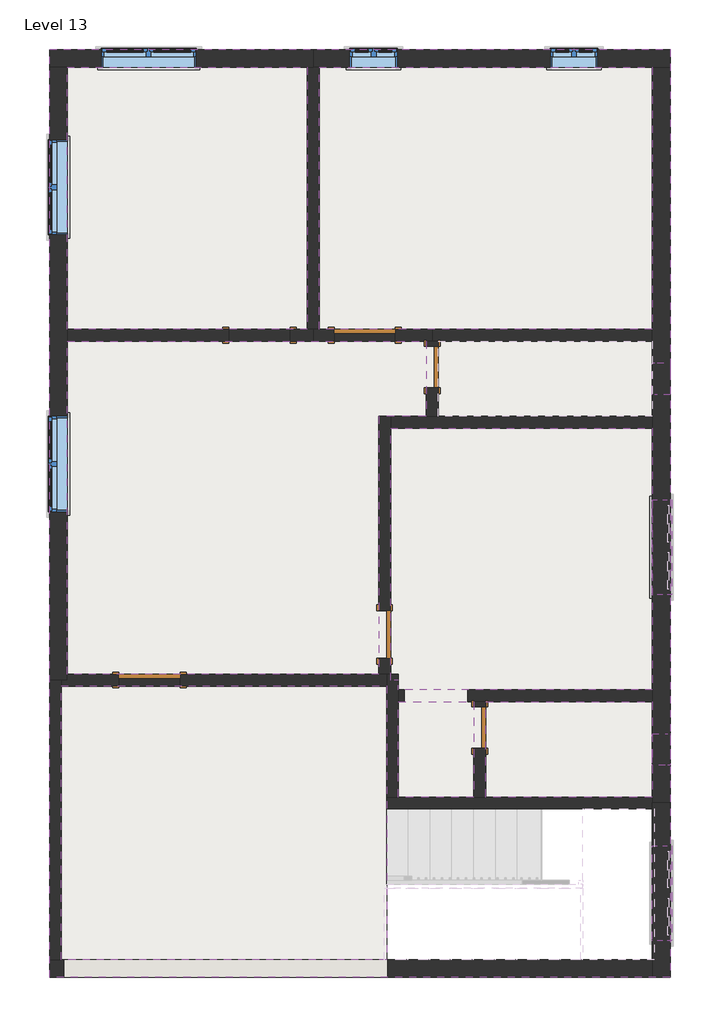
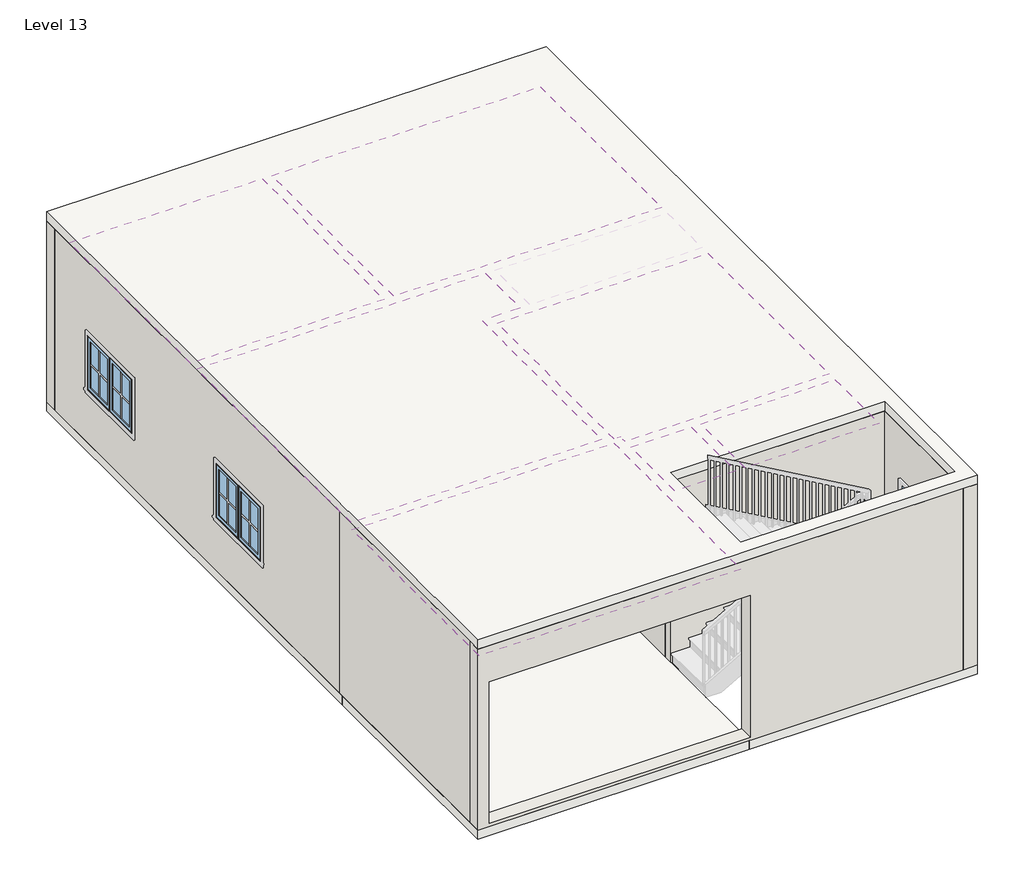
# One storey, part 1 of 2: 27 walls, 13 windows, 7 coverings, 6 doors, 3 slabs.
# Revit data of these elements (continued)
# Element 47 (IfcWindow, "Window-Casement-Double : 3'") (continued)
#   Materials on its faces: "Wood - Stained", "Glass", "Clad - White"
# Element 48 (IfcWindow, "Window-Casement-Double : 3'")
#   Mark = "38"
#   Window Inset = 0' - 0"
#   Interior Wall Closure = 0' - 2 1/4"
#   Frame Extension = 0' - 0 1/4"
#   Exterior Wall Closure = 0' - 1 1/4"
#   Interior Trim Visibility = yes
#   Exterior Trim Visibility = yes
#   Phase Created = New Construction
#   Materials on its faces: "Wood - Stained", "Glass", "Clad - White"
# Element 49 (IfcWindow, "Window-Casement-Double : 3'")
#   Mark = "39"
#   Window Inset = 0' - 0"
#   Interior Wall Closure = 0' - 2 1/4"
#   Frame Extension = 0' - 0 1/4"
#   Exterior Wall Closure = 0' - 1 1/4"
#   Interior Trim Visibility = yes
#   Exterior Trim Visibility = yes
#   Phase Created = New Construction
#   Materials on its faces: "Wood - Stained", "Glass", "Clad - White"
# Element 50 (IfcWindow, "Window-Casement-Double : 4'")
#   Mark = "27"
#   Window Inset = 0' - 0"
#   Interior Wall Closure = 0' - 2 1/4"
#   Frame Extension = 0' - 0 1/4"
#   Exterior Wall Closure = 0' - 1 1/4"
#   Interior Trim Visibility = yes
#   Exterior Trim Visibility = yes
#   Phase Created = New Construction
#   Materials on its faces: "Wood - Stained", "Glass", "Clad - White"
# Element 51 (IfcWindow, "Window-Casement-Double : 4'")
#   Mark = "28"
#   Window Inset = 0' - 0"
#   Interior Wall Closure = 0' - 2 1/4"
#   Frame Extension = 0' - 0 1/4"
#   Exterior Wall Closure = 0' - 1 1/4"
#   Interior Trim Visibility = yes
#   Exterior Trim Visibility = yes
#   Phase Created = New Construction
#   Materials on its faces: "Wood - Stained", "Glass", "Clad - White"
# Element 52 (IfcWindow, "Window-Casement-Double : 4'")
#   Mark = "29"
#   Window Inset = 0' - 0"
#   Interior Wall Closure = 0' - 2 1/4"
#   Frame Extension = 0' - 0 1/4"
#   Exterior Wall Closure = 0' - 1 1/4"
#   Interior Trim Visibility = yes
#   Exterior Trim Visibility = yes
#   Phase Created = New Construction
#   Materials on its faces: "Wood - Stained", "Glass", "Clad - White"
# Element 53 (IfcWindow, "Window-Casement-Double : 4'")
#   Mark = "30"
#   Window Inset = 0' - 0"
#   Interior Wall Closure = 0' - 2 1/4"
#   Frame Extension = 0' - 0 1/4"
#   Exterior Wall Closure = 0' - 1 1/4"
#   Interior Trim Visibility = yes
#   Exterior Trim Visibility = yes
#   Phase Created = New Construction
#   Materials on its faces: "Wood - Stained", "Glass", "Clad - White"
# Element 54 (IfcWindow, "Window-Casement-Double : 4'")
#   Mark = "31"
#   Window Inset = 0' - 0"
#   Interior Wall Closure = 0' - 2 1/4"
#   Frame Extension = 0' - 0 1/4"
#   Exterior Wall Closure = 0' - 1 1/4"
#   Interior Trim Visibility = yes
#   Exterior Trim Visibility = yes
#   Phase Created = New Construction
#   Materials on its faces: "Wood - Stained", "Glass", "Clad - White"
# Element 55 (IfcWindow, "Window-Casement-Double : 4'")
#   Mark = "36"
#   Window Inset = 0' - 0"
#   Interior Wall Closure = 0' - 2 1/4"
#   Frame Extension = 0' - 0 1/4"
#   Exterior Wall Closure = 0' - 1 1/4"
#   Interior Trim Visibility = yes
#   Exterior Trim Visibility = yes
#   Phase Created = New Construction
#   Materials on its faces: "Wood - Stained", "Glass", "Clad - White"
# Element 56 (IfcWindow, "Window-Casement-Double : 4'")
#   Mark = "37"
#   Window Inset = 0' - 0"
#   Interior Wall Closure = 0' - 2 1/4"
#   Frame Extension = 0' - 0 1/4"
#   Exterior Wall Closure = 0' - 1 1/4"
#   Interior Trim Visibility = yes
#   Exterior Trim Visibility = yes
#   Phase Created = New Construction
#   Materials on its faces: "Wood - Stained", "Glass", "Clad - White"
# Materials
#   "Default": colour RGB 127 127 127, transparency 0, Cost = 0
#   "Acoustic Ceiling Tile 24 x 48": class "Generic", colour RGB 229 229 229, transparency 0, Description = "Acoustic Ceiling Tile 24 x 48", Cost = 0
#   "Door - Panel": class "Wood", colour RGB 210 159 95, transparency 0, Cost = 0
#   "Door - Frame": colour RGB 118 70 51, transparency 0, Cost = 0
#   "Glass": class "Glass", colour RGB 0 128 192, transparency 0.75, Description = "Soda Lime Glass", Cost = 0
#   "Sash": class "Wood", colour RGB 224 178 126, transparency 0, Cost = 0
#   "Wood - Stained": class "Wood", colour RGB 224 178 126, transparency 0, Cost = 0
#   "Clad - White": class "Wood", colour RGB 242 242 238, transparency 0, Cost = 0
#   "Default Floor": colour RGB 128 128 128, transparency 0, Cost = 0
#   "TILE": class "Generic", colour RGB 120 120 120, transparency 0, Cost = 0
#   "Grass": class "Generic", colour RGB 104 137 66, transparency 0, Description = "Physical material.", Cost = 0
#   "Default Wall": colour RGB 128 128 128, transparency 0, Cost = 0
#   "WALL PAINT 4": class "Generic", colour RGB 120 120 120, transparency 0, Cost = 0
#   "MARBLE": class "Generic", colour RGB 120 120 120, transparency 0, Cost = 0
#   "WALL PAINT 5": class "Generic", colour RGB 120 120 120, transparency 0, Cost = 0
#   "WALL PAINT 2": class "Generic", colour RGB 120 120 120, transparency 0, Cost = 0
#   "WALL PAINT 3": class "Generic", colour RGB 120 120 120, transparency 0, Cost = 0
#   "WALL PAINT 1": class "Generic", colour RGB 120 120 120, transparency 0, Cost = 0
